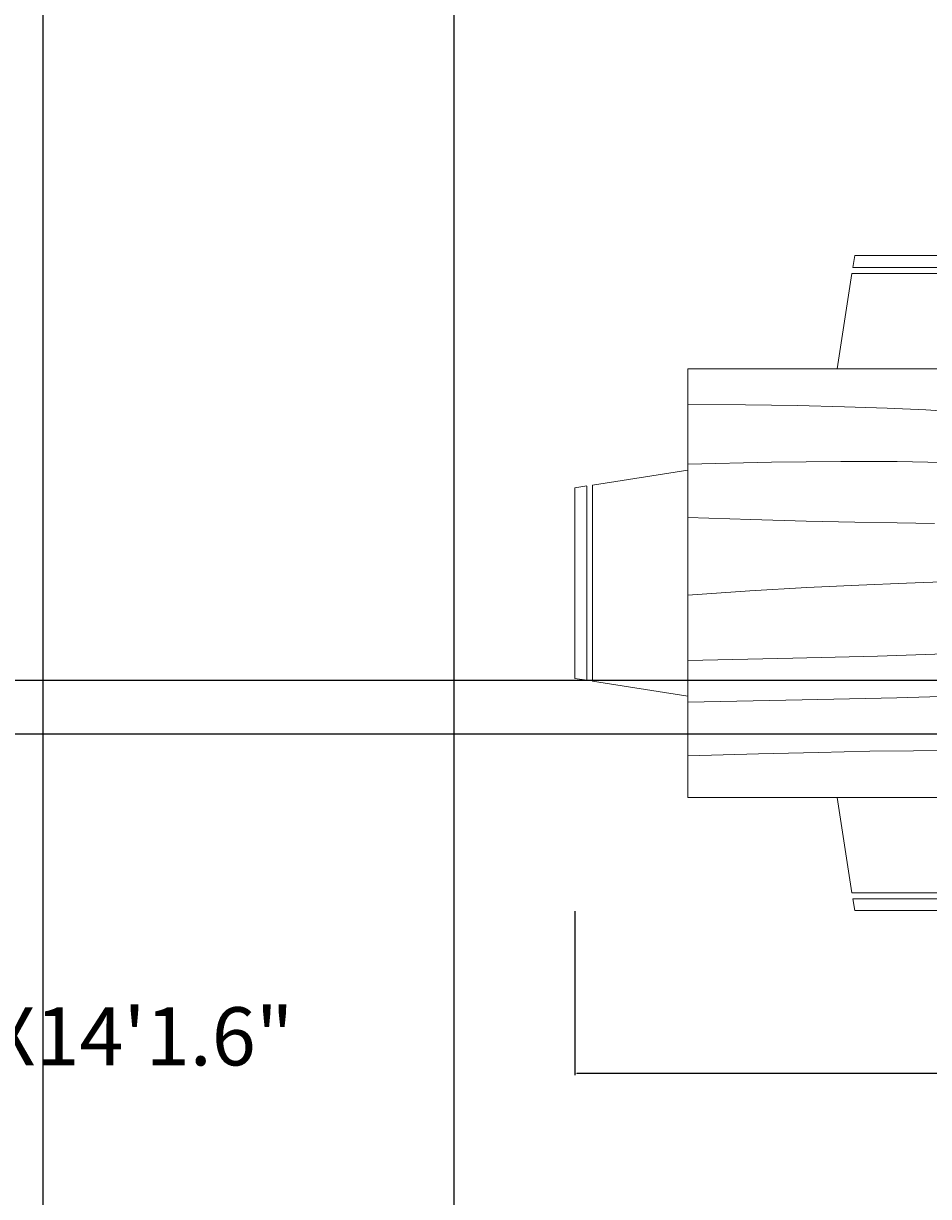
# Model space of a CAD drawing. Units: inches. Extents: x 7359 to 7979, y 33027 to 34263.
# Tile 6 of 32: x 7612 to 7688, y 33347 to 33446. Entities that reach past the tile are written whole.
import ezdxf

# ---------------------------------------------------------------- set-up
doc = ezdxf.new("R2010")
doc.units = ezdxf.units.IN
for name, color, linetype, lineweight in [('A-ANNO-DIMS', 2, 'Continuous', 18), ('A-AREA-IDEN', 7, 'Continuous', 18), ('A-FURN', 8, 'Continuous', 18)]:
    doc.layers.add(name, color=color, linetype=linetype, lineweight=lineweight)
doc.styles.get("Standard").update_dxf_attribs({"font": 'arial.ttf'})
doc.dimstyles.get("Standard").update_dxf_attribs({"dimtxt": 0.18, "dimasz": 0.18, "dimexe": 0.18, "dimexo": 0.0625, "dimgap": 0.09, "dimtad": 0, "dimtih": 1, "dimtoh": 1, "dimdec": 4, "dimzin": 0, "dimdsep": 46, "dimtxsty": 'Standard', "dimcen": 0.09, "dimadec": 0, "dimazin": 0, "dimtfac": 1, "dimtdec": 4, "dimtofl": 0, "dimtmove": 0, "dimatfit": 3, "dimfxl": 1, "dimtolj": 1, "dimtzin": 0, "dimarcsym": 0})

# ---------------------------------------------------------------- blocks, each defined once
blk = doc.blocks.new('Dining Set - 36 x 72 in.')
for p, q in [((-22, 27.5), (-22.1562, 26.50042)), ((-22, 27.5), (-6, 27.5)), ((-22.2343, 26.00059), (-23.4847, 17.99762)), ((-22.2304, 26), (-5.7608, 26)), ((-5.8416, 26.5), (-22.1534, 26.5)), ((36, 18), (-36, 18)), ((-36, 18), (-36, -18)), ((-44.0006, 8.23428), (-35.9976, 9.48474)), ((-45.5, 8), (-44.5004, 8.15617)), ((-45.5, 8), (-45.5, -8)), ((-44.5, -8.15843), (-44.5, 8.15338)), ((-44, 8.23041), (-44, -8.23915)), ((-44.4997, -8.15631), (-45.5, -8)), ((-35.9976, -9.48476), (-43.9993, -8.2345)), ((-36, -18), (36, -18)), ((-22.2343, -26.0006), (-23.4847, -17.99762)), ((-22.2304, -26), (-5.7608, -26)), ((-22, -27.5), (-22.1562, -26.50044)), ((-5.8416, -26.5), (-22.1534, -26.5)), ((-22, -27.5), (-6, -27.5))]:
    blk.add_line(p, q)
for points in [[(-36, 15), (-31.1772, 14.97754), (-26.8079, 14.91406), (-22.8538, 14.81543), (-19.276, 14.6875), (-16.0362, 14.53613), (-13.0957, 14.36718)], [(-36, 10), (-28.9766, 10.14274), (-23.1725, 10.20442), (-18.4241, 10.19775), (-14.5677, 10.13541)], [(-36, 5.5), (-30.7157, 5.3348), (-26.069, 5.20963), (-21.9946, 5.11767), (-18.4271, 5.05208), (-15.3009, 5.00602)], [(-36, -1), (-30.7915, -0.6591), (-26.0195, -0.38216), (-21.6519, -0.16284), (-17.6563, 0.00521), (-14.0005, 0.12833)], [(-36, -6.5), (-27.1843, -6.31267), (-20.084, -6.1263), (-14.469, -5.9419)], [(-36, -10), (-26.4022, -9.81299), (-18.4675, -9.62891), (-11.9839, -9.45069)], [(-36, -14.5), (-30.0881, -14.33513), (-25.0332, -14.21224), (-20.7312, -14.12647), (-17.0781, -14.07292), (-13.97, -14.04671)]]:
    blk.add_lwpolyline(points)
blk = doc.blocks.new('*D36')
at = {"layer": 'A-ANNO-DIMS', "color": 0, "lineweight": -2, "transparency": 16777216}
for p, q in [((7657.863, 33371.281), (7657.863, 33357.514)), ((7748.863, 33371.281), (7748.863, 33357.514)), ((7658.043, 33357.694), (7702.085, 33357.694)), ((7748.683, 33357.694), (7704.641, 33357.694))]:
    blk.add_line(p, q, dxfattribs=at)
at = {"layer": 'A-ANNO-DIMS', "color": 0, "transparency": 16777216}
for points in [[(7658.043, 33357.724), (7658.043, 33357.664), (7657.863, 33357.694)], [(7748.683, 33357.724), (7748.683, 33357.664), (7748.863, 33357.694)]]:
    blk.add_solid(points, dxfattribs=at)
at = {"layer": 'Defpoints', "color": 0, "transparency": 16777216}
for p in [(7657.863, 33371.344), (7748.863, 33371.344), (7748.863, 33357.694)]:
    blk.add_point(p, dxfattribs=at)
at = {"layer": 'A-ANNO-DIMS', "color": 0, "transparency": 16777216, "insert": (7703.363, 33357.694), "char_height": 0.18, "attachment_point": 5}
blk.add_mtext('\\A1;DINING SET 91 TYP.', dxfattribs=at)
blk = doc.blocks.new('*D73')
at = {"layer": 'A-ANNO-DIMS', "color": 0, "lineweight": -2, "transparency": 16777216}
for p, q in [((7613.227, 33618.1), (7613.227, 33027.177)), ((7647.706, 33618.1), (7647.706, 33027.177)), ((7613.407, 33027.357), (7630.073, 33027.357)), ((7647.526, 33027.357), (7630.86, 33027.357))]:
    blk.add_line(p, q, dxfattribs=at)
at = {"layer": 'A-ANNO-DIMS', "color": 0, "transparency": 16777216}
for points in [[(7613.407, 33027.387), (7613.407, 33027.327), (7613.227, 33027.357)], [(7647.526, 33027.387), (7647.526, 33027.327), (7647.706, 33027.357)]]:
    blk.add_solid(points, dxfattribs=at)
at = {"layer": 'Defpoints', "color": 0, "transparency": 16777216}
for p in [(7613.227, 33618.162), (7647.706, 33618.162), (7647.706, 33027.357)]:
    blk.add_point(p, dxfattribs=at)
at = {"layer": 'A-ANNO-DIMS', "color": 0, "transparency": 16777216, "insert": (7630.466, 33027.357), "char_height": 0.18, "attachment_point": 5}
blk.add_mtext('\\A1;34.48', dxfattribs=at)
blk = doc.blocks.new('*D85')
at = {"layer": 'A-ANNO-DIMS', "color": 0, "lineweight": -2, "transparency": 16777216}
for p, q in [((7793.064, 33390.662), (7369.542, 33390.662)), ((7369.722, 33390.482), (7369.722, 33388.594)), ((7369.722, 33386.342), (7369.722, 33388.231)), ((7793.064, 33386.162), (7369.542, 33386.162))]:
    blk.add_line(p, q, dxfattribs=at)
at = {"layer": 'A-ANNO-DIMS', "color": 0, "transparency": 16777216}
for points in [[(7369.692, 33390.482), (7369.752, 33390.482), (7369.722, 33390.662)], [(7369.692, 33386.342), (7369.752, 33386.342), (7369.722, 33386.162)]]:
    blk.add_solid(points, dxfattribs=at)
at = {"layer": 'Defpoints', "color": 0, "transparency": 16777216}
for p in [(7793.127, 33390.662), (7369.722, 33386.162), (7793.127, 33386.162)]:
    blk.add_point(p, dxfattribs=at)
at = {"layer": 'A-ANNO-DIMS', "color": 0, "transparency": 16777216, "insert": (7369.722, 33388.412), "char_height": 0.18, "attachment_point": 5}
blk.add_mtext('\\A1;4.5', dxfattribs=at)

msp = doc.modelspace()

# ---------------------------------------------------------------- block references
at = {"layer": 'A-FURN'}
msp.add_blockref('Dining Set - 36 x 72 in.', (7703.363, 33398.8436), dxfattribs=at)

# ---------------------------------------------------------------- texts
at = {"layer": 'A-AREA-IDEN'}
msp.add_text('25\'10.9"X14\'1.6"', height=4.885549, dxfattribs=at).set_placement((7583.409, 33358.3411))

# ---------------------------------------------------------------- dimensions: what is measured, and where the dimension line sits
at = {"layer": 'A-ANNO-DIMS'}
dim = msp.add_linear_dim(base=(7647.7062, 33027.3568), p1=(7613.2266, 33618.1623), p2=(7647.7062, 33618.1623), dimstyle='Standard', override={"dimdec": 2, "dimlfac": 1, "dimrnd": 0, "dimzin": 0, "dimdsep": 46, "dimlunit": 2}, dxfattribs=at)
dim.commit()
dim.dimension.update_dxf_attribs({"geometry": '*D73', "text_midpoint": (7630.4664, 33027.3568)})
dim = msp.add_linear_dim(base=(7369.7217, 33386.1623), p1=(7793.1266, 33390.6623), p2=(7793.1266, 33386.1623), angle=90, dimstyle='Standard', override={"dimdec": 1, "dimlfac": 1, "dimrnd": 0, "dimzin": 0, "dimdsep": 46, "dimlunit": 2}, dxfattribs=at)
dim.commit()
dim.dimension.update_dxf_attribs({"geometry": '*D85', "text_midpoint": (7369.7217, 33388.4123)})
dim = msp.add_linear_dim(base=(7748.863, 33357.6936), p1=(7657.863, 33371.3436), p2=(7748.863, 33371.3436), text='DINING SET <> TYP.', dimstyle='Standard', override={"dimdec": 0, "dimlfac": 1, "dimrnd": 0, "dimzin": 0, "dimdsep": 46, "dimlunit": 2}, dxfattribs=at)
dim.commit()
dim.dimension.update_dxf_attribs({"geometry": '*D36', "text_midpoint": (7703.363, 33357.6936)})

doc.saveas('drawing.dxf')
